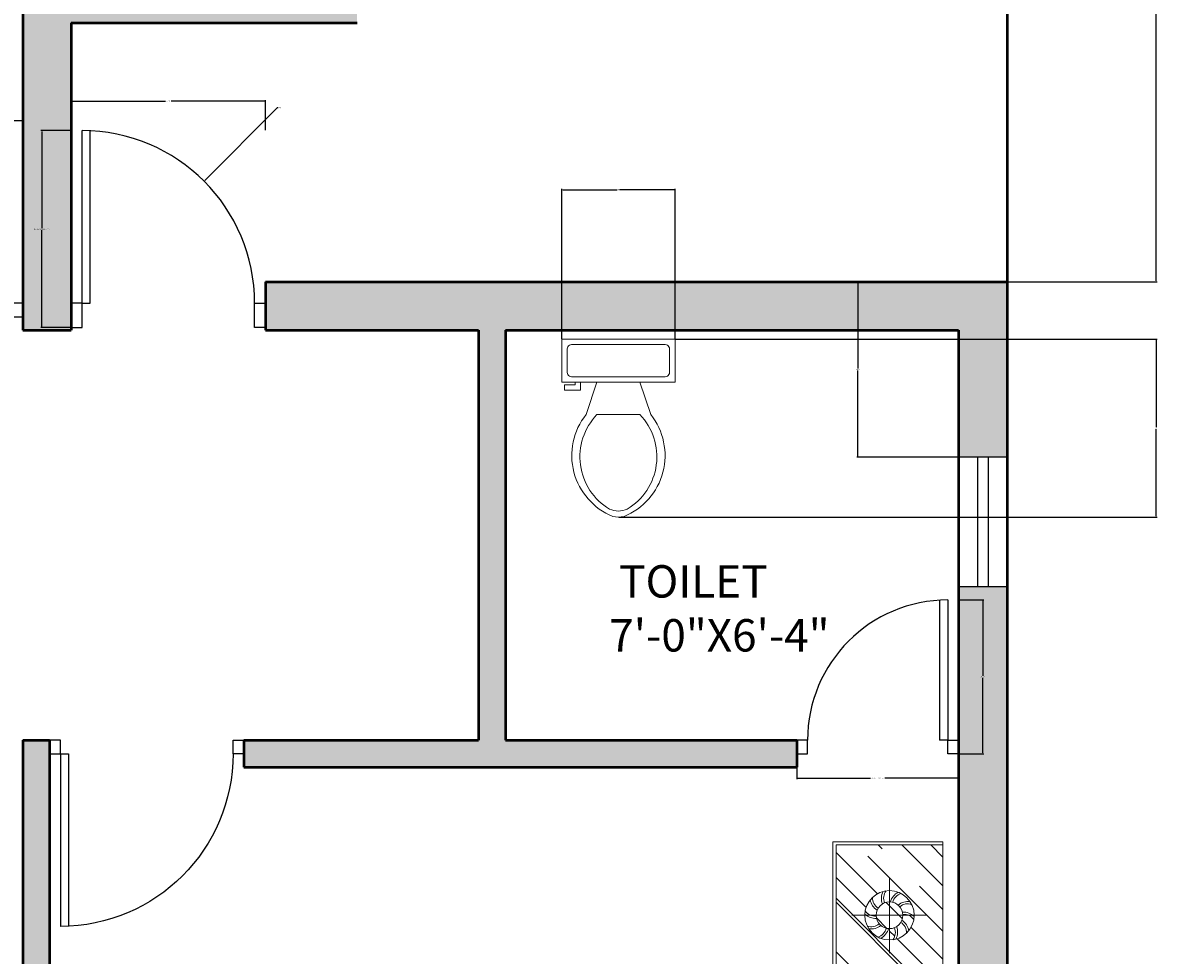
# Model space of a CAD drawing. Units: inches. Extents: x 2831 to 3729, y 3926 to 4974.
# Tile 7 of 8: x 3519 to 3729, y 4672 to 4845. Entities that reach past the tile are written whole.
import ezdxf

# ---------------------------------------------------------------- set-up
doc = ezdxf.new("R2010")
doc.units = ezdxf.units.IN
for name, color, linetype, lineweight in [('A-ANNO-DIMS', 2, 'Continuous', 18), ('A-AREA-IDEN', 7, 'Continuous', 18), ('A-DOOR', 3, 'Continuous', 25), ('A-FLOR-FIXT', 9, 'Continuous', 18), ('A-FURN', 8, 'Continuous', 18), ('A-GLAZ', 4, 'Continuous', 25), ('A-WALL', 7, 'Continuous', 50), ('A-WALL-PATT', 252, 'Continuous', 13)]:
    doc.layers.add(name, color=color, linetype=linetype, lineweight=lineweight)
doc.styles.get("Standard").update_dxf_attribs({"font": 'arial.ttf'})
doc.dimstyles.get("Standard").update_dxf_attribs({"dimtxt": 0.18, "dimasz": 0.18, "dimexe": 0.18, "dimexo": 0.0625, "dimgap": 0.09, "dimtad": 0, "dimtih": 1, "dimtoh": 1, "dimdec": 4, "dimzin": 0, "dimdsep": 46, "dimtxsty": 'Standard', "dimcen": 0.09, "dimadec": 0, "dimazin": 0, "dimtfac": 1, "dimtdec": 4, "dimtofl": 0, "dimtmove": 0, "dimatfit": 3, "dimfxl": 1, "dimtolj": 1, "dimtzin": 0, "dimarcsym": 0})

# ---------------------------------------------------------------- blocks, each defined once
blk = doc.blocks.new('A$C64B41DC1')
for p, q in [((0, 2.5079), (2.9903, 2.5079)), ((0, 2.0879), (0, 2.5079)), ((0.012, 2.4618), (0.0581, 2.5079)), ((0.012, 2.3515), (0.1684, 2.5079)), ((0.012, 2.0999), (0.012, 2.5079)), ((0.0543, 2.2213), (0.3409, 2.5079)), ((0.1689, 2.4179), (0.2589, 2.5079)), ((0.3265, 2.386), (0.4484, 2.5079)), ((0.3699, 2.3332), (0.5445, 2.5079)), ((0.548, 2.5079), (0.548, 2.0999)), ((0.56, 2.5079), (0.56, 2.0879)), ((0.6301, 2.5079), (0.6301, 0.4779)), ((0.6401, 2.461), (0.6401, 2.5079)), ((0.6401, 2.5079), (2.344, 2.5079)), ((2.344, 2.5079), (2.3601, 2.5079)), ((2.344, 2.5079), (2.344, 2.461)), ((2.3601, 2.5079), (2.3601, 2.4761)), ((2.3601, 0.4779), (2.3601, 2.5079)), ((2.4303, 2.5079), (2.4303, 2.0879)), ((2.4423, 2.5079), (2.4423, 2.0999)), ((2.4423, 2.3333), (2.6169, 2.5079)), ((2.4423, 2.2145), (2.7357, 2.5079)), ((2.4423, 2.404), (2.5354, 2.4971)), ((2.705, 2.398), (2.8149, 2.5079)), ((2.7691, 2.3772), (2.8998, 2.5079)), ((2.7819, 2.3646), (2.9252, 2.5079)), ((2.9783, 2.0999), (2.9783, 2.5079)), ((2.9903, 2.0879), (2.9903, 2.5079)), ((0.2157, 2.0999), (0.548, 2.4322)), ((0.2804, 2.1597), (0.2804, 2.4481)), ((2.344, 2.461), (0.6401, 2.461)), ((0.6601, 2.4461), (1.4951, 2.4461)), ((0.6601, 2.4461), (0.6601, 0.5579)), ((1.4951, 2.4461), (0.6697, 2.4461)), ((2.3301, 2.4461), (1.4951, 2.4461)), ((2.3301, 0.5579), (2.3301, 2.4461)), ((2.7099, 2.1597), (2.7099, 2.4481)), ((0.2299, 2.0999), (0.548, 2.418)), ((0.2311, 2.2906), (0.2937, 2.3532)), ((2.6674, 2.2756), (2.7382, 2.3464)), ((2.7914, 2.1846), (2.9783, 2.3715)), ((0.1362, 2.3039), (0.4246, 2.3039)), ((0.3405, 2.3039), (0.3605, 2.3238)), ((2.8541, 2.3039), (2.5657, 2.3039)), ((2.5849, 2.2779), (2.6158, 2.3088)), ((2.6158, 2.3088), (2.6313, 2.3243)), ((2.7249, 2.3076), (2.7512, 2.3339)), ((2.7746, 2.0999), (2.9783, 2.3036)), ((0.012, 2.261), (0.0275, 2.2765)), ((0.0404, 2.0999), (0.1982, 2.2578)), ((0.2905, 2.2539), (0.3304, 2.2938)), ((2.9144, 2.2312), (2.9783, 2.2951)), ((0.1365, 2.0999), (0.251, 2.2144)), ((0.4194, 2.0999), (0.548, 2.2285)), ((2.4423, 2.1353), (2.5382, 2.2312)), ((2.4918, 2.0999), (2.6366, 2.2447)), ((2.7831, 2.0999), (2.8678, 2.1846)), ((2.8962, 2.0999), (2.9783, 2.182)), ((0.4986, 2.0999), (0.548, 2.1493)), ((0.5127, 2.0999), (0.548, 2.1352)), ((0.56, 2.0879), (0, 2.0879)), ((0.548, 2.0999), (0.012, 2.0999)), ((2.4303, 2.0879), (2.9903, 2.0879)), ((2.4423, 2.0999), (2.9783, 2.0999)), ((2.5172, 2.0999), (2.5269, 2.1096)), ((0.9415, 1.9902), (0.9415, 1.3975)), ((0.9715, 1.9906), (0.9715, 1.4076)), ((1.0015, 1.991), (1.0015, 1.4177)), ((1.0315, 1.9916), (1.0315, 1.4279)), ((2.3349, 1.8678), (0.6613, 1.3029)), ((0.8956, 1.1191), (2.3349, 1.8678)), ((1.6636, 1.6412), (0.6601, 1.6412)), ((1.5748, 1.6112), (0.6601, 1.6112)), ((2.377, 1.295), (2.3822, 1.3891)), ((2.4451, 1.295), (2.4503, 1.3891)), ((2.5105, 1.295), (2.5157, 1.3891)), ((2.5471, 1.295), (2.5524, 1.3891)), ((2.7043, 1.295), (2.7095, 1.3891)), ((2.8653, 1.2966), (2.8688, 1.3861)), ((2.3665, 1.295), (2.3665, 1.3839)), ((2.4032, 1.295), (2.4032, 1.3839)), ((2.4346, 1.295), (2.4346, 1.3839)), ((2.4774, 1.2957), (2.4774, 1.3837)), ((2.5, 1.295), (2.5, 1.3839)), ((2.5367, 1.295), (2.5367, 1.3839)), ((2.5681, 1.295), (2.5681, 1.3839)), ((2.5918, 1.295), (2.5918, 1.3839)), ((2.6346, 1.2957), (2.6346, 1.3837)), ((2.6362, 1.2957), (2.6467, 1.3839)), ((2.6729, 1.295), (2.6624, 1.3839)), ((2.6938, 1.295), (2.6938, 1.3839)), ((2.7127, 1.2957), (2.7232, 1.3839)), ((2.7253, 1.295), (2.7253, 1.3839)), ((2.7494, 1.295), (2.7389, 1.3839)), ((2.7718, 1.295), (2.7718, 1.3839)), ((2.7959, 1.295), (2.7854, 1.3839)), ((2.8146, 1.2957), (2.8146, 1.3837)), ((2.8146, 1.2957), (2.8146, 1.3837)), ((2.8282, 1.295), (2.8282, 1.3839)), ((2.8282, 1.295), (2.8282, 1.3839)), ((2.8523, 1.295), (2.8418, 1.3839)), ((2.8523, 1.295), (2.8418, 1.3839)), ((2.8711, 1.2957), (2.8711, 1.3837)), ((2.8711, 1.2957), (2.8875, 1.3822)), ((2.8765, 1.2958), (2.9132, 1.3758)), ((2.8893, 1.3011), (2.9394, 1.3636)), ((2.8713, 1.2927), (2.954, 1.3315)), ((2.8717, 1.2884), (2.9588, 1.3058)), ((2.3601, 1.2873), (2.8639, 1.2873)), ((2.8639, 1.2873), (2.8639, 0.1018)), ((2.8716, 1.2565), (2.9605, 1.2669)), ((2.8744, 1.2817), (2.9603, 1.2869)), ((2.3601, 1.2233), (2.7999, 1.2233)), ((2.7999, 1.2233), (2.7999, 0.1658)), ((2.8716, 1.2212), (2.9605, 1.2212)), ((2.8723, 1.2489), (2.9603, 1.2489)), ((2.3601, 1.1913), (2.7679, 1.1912)), ((2.7679, 1.1912), (2.7679, 0.1978)), ((2.8716, 1.1947), (2.9605, 1.2052)), ((2.8716, 1.181), (2.9605, 1.1705)), ((2.8723, 1.1872), (2.9603, 1.1872)), ((2.8716, 1.1595), (2.9605, 1.1595)), ((2.8716, 1.133), (2.9605, 1.1435)), ((2.8716, 1.1193), (2.9605, 1.1088)), ((2.8716, 1.1035), (2.9605, 1.093)), ((2.8716, 1.0965), (2.9605, 1.0965)), ((2.8716, 1.086), (2.9657, 1.0913)), ((2.8723, 1.1255), (2.9603, 1.1255)), ((2.8723, 1.0858), (2.9605, 1.0753)), ((2.8716, 1.0756), (2.9605, 1.0756)), ((2.8716, 1.0491), (2.9605, 1.0596)), ((2.8723, 1.0416), (2.9603, 1.0416)), ((2.8716, 1.0354), (2.9605, 1.0249)), ((2.8723, 0.9987), (2.9605, 1.0092)), ((2.8723, 0.985), (2.9605, 0.9745)), ((2.8723, 0.9735), (2.9603, 0.9735)), ((2.8716, 0.9346), (2.9605, 0.9241)), ((2.8723, 0.9408), (2.9603, 0.9408)), ((2.8723, 0.8979), (2.9605, 0.9084)), ((2.8723, 0.8726), (2.9603, 0.8726)), ((2.8723, 0.8505), (2.9603, 0.8505)), ((2.8716, 0.7885), (2.9605, 0.799)), ((2.8716, 0.7818), (2.9657, 0.787)), ((2.8716, 0.7503), (2.9657, 0.7556)), ((2.8723, 0.7571), (2.9605, 0.7466)), ((2.8716, 0.7204), (2.9605, 0.7309)), ((2.8716, 0.6995), (2.9605, 0.6995)), ((2.8716, 0.689), (2.9657, 0.6838)), ((2.8716, 0.6576), (2.9657, 0.6523)), ((2.8716, 0.6471), (2.9605, 0.6471)), ((2.8716, 0.5903), (2.9605, 0.6007)), ((2.882, 0.5582), (2.9657, 0.5536)), ((2.8909, 0.5263), (2.9657, 0.5222)), ((0.6301, 0.4779), (2.3601, 0.4779)), ((0.7101, 0.5079), (2.2801, 0.5079)), ((1.2542, 0.1018), (1.2542, 0.4779)), ((1.3182, 0.1658), (1.3182, 0.4779)), ((1.3502, 0.1978), (1.3502, 0.4779)), ((2.8716, 0.4877), (2.9603, 0.4877)), ((2.8928, 0.5169), (2.9605, 0.5169)), ((1.2465, 0.4625), (1.1576, 0.452)), ((1.2465, 0.4365), (1.1577, 0.4365)), ((2.8716, 0.4625), (2.9605, 0.452)), ((2.8716, 0.4365), (2.9603, 0.4365)), ((1.2465, 0.3746), (1.1576, 0.3851)), ((1.2465, 0.3684), (1.1577, 0.3684)), ((2.8716, 0.3746), (2.9605, 0.3851)), ((2.8716, 0.3684), (2.9603, 0.3684)), ((1.2355, 0.3092), (1.1576, 0.3)), ((1.2285, 0.3357), (1.1577, 0.3357)), ((2.8826, 0.3092), (2.9605, 0.3)), ((2.8896, 0.3357), (2.9603, 0.3357)), ((1.2457, 0.2676), (1.1577, 0.2676)), ((2.8723, 0.2676), (2.9603, 0.2676)), ((1.2457, 0.2423), (1.1576, 0.2319)), ((2.8723, 0.2423), (2.9605, 0.2319)), ((1.2465, 0.1742), (1.1524, 0.169)), ((1.2465, 0.2057), (1.1576, 0.2161)), ((1.2465, 0.1847), (1.1576, 0.1847)), ((2.7679, 0.1978), (1.3502, 0.1978)), ((2.8716, 0.2057), (2.9605, 0.2161)), ((2.8716, 0.1847), (2.9605, 0.1847)), ((2.8716, 0.1742), (2.9657, 0.169)), ((1.2465, 0.1428), (1.1524, 0.1376)), ((1.2465, 0.1334), (1.1524, 0.1281)), ((1.2465, 0.1323), (1.1576, 0.1323)), ((1.2465, 0.1323), (1.1576, 0.1323)), ((2.7999, 0.1658), (1.3182, 0.1658)), ((2.8716, 0.1428), (2.9657, 0.1376)), ((2.8716, 0.1334), (2.9657, 0.1281)), ((2.8716, 0.1323), (2.9605, 0.1323)), ((1.2465, 0.1), (1.1576, 0.1105)), ((1.2465, 0.1229), (1.1588, 0.1168)), ((1.2464, 0.1007), (1.1592, 0.0833)), ((1.2468, 0.0964), (1.1641, 0.0576)), ((1.2288, 0.088), (1.1787, 0.0255)), ((1.2415, 0.0933), (1.2049, 0.0133)), ((1.247, 0.0934), (1.2306, 0.0069)), ((1.2527, 0.0925), (1.2493, 0.003)), ((2.8639, 0.1018), (1.2542, 0.1018)), ((1.2658, 0.0941), (1.2762, 0.0052)), ((1.2899, 0.0941), (1.2899, 0.0052)), ((1.2999, 0.0941), (1.3051, 0)), ((1.3313, 0.0941), (1.3365, 0)), ((1.3523, 0.0941), (1.3575, 0)), ((1.3804, 0.0941), (1.3699, 0.0052)), ((1.4119, 0.0934), (1.4223, 0.0052)), ((1.4485, 0.0941), (1.438, 0.0052)), ((1.48, 0.0941), (1.4852, 0)), ((1.5114, 0.0941), (1.5166, 0)), ((1.5323, 0.0941), (1.5376, 0)), ((1.5638, 0.0941), (1.5638, 0.0105)), ((1.6021, 0.0941), (1.6021, 0.0052)), ((1.6336, 0.0941), (1.6336, 0.0052)), ((1.6702, 0.0941), (1.6702, 0.0052)), ((1.7017, 0.0941), (1.7017, 0.0052)), ((1.7122, 0.0941), (1.7174, 0)), ((1.7445, 0.0934), (1.7445, 0.0054)), ((1.7698, 0.0934), (1.7803, 0.0052)), ((1.8065, 0.0941), (1.796, 0.0052)), ((1.8274, 0.0941), (1.8274, 0.0052)), ((1.8379, 0.0941), (1.8431, 0)), ((1.8746, 0.0941), (1.8798, 0)), ((1.8955, 0.0941), (1.8955, 0.0052)), ((1.906, 0.0941), (1.9113, 0)), ((1.9384, 0.0934), (1.9384, 0.0054)), ((1.9609, 0.0941), (1.9609, 0.0052)), ((1.9636, 0.0934), (1.9741, 0.0052)), ((1.9714, 0.0941), (1.9766, 0)), ((1.9976, 0.0941), (1.9976, 0.0052)), ((2.0081, 0.0941), (2.0133, 0)), ((2.029, 0.0941), (2.029, 0.0052)), ((2.0395, 0.0941), (2.0447, 0)), ((2.0797, 0.0941), (2.0797, 0.0052)), ((2.0902, 0.0941), (2.0954, 0)), ((2.1216, 0.0941), (2.1269, 0)), ((2.1412, 0.0941), (2.1412, 0.0052)), ((2.1517, 0.0941), (2.1569, 0)), ((2.1831, 0.0941), (2.1884, 0)), ((2.2093, 0.0941), (2.2093, 0.0052)), ((2.2198, 0.0941), (2.225, 0)), ((2.2512, 0.0941), (2.2565, 0)), ((2.2603, 0.0934), (2.2707, 0.0052)), ((2.2969, 0.0941), (2.2864, 0.0052)), ((2.3089, 0.0934), (2.3193, 0.0052)), ((2.3455, 0.0941), (2.3351, 0.0052)), ((2.3665, 0.0941), (2.3665, 0.0052)), ((2.377, 0.0941), (2.3822, 0)), ((2.4032, 0.0941), (2.4032, 0.0052)), ((2.4346, 0.0941), (2.4346, 0.0052)), ((2.4451, 0.0941), (2.4503, 0)), ((2.4774, 0.0934), (2.4774, 0.0054)), ((2.5, 0.0941), (2.5, 0.0052)), ((2.5105, 0.0941), (2.5157, 0)), ((2.5367, 0.0941), (2.5367, 0.0052)), ((2.5471, 0.0941), (2.5524, 0)), ((2.5681, 0.0941), (2.5681, 0.0052)), ((2.5918, 0.0941), (2.5918, 0.0052)), ((2.6346, 0.0934), (2.6346, 0.0054)), ((2.6362, 0.0934), (2.6467, 0.0052)), ((2.6729, 0.0941), (2.6624, 0.0052)), ((2.6938, 0.0941), (2.6938, 0.0052)), ((2.7043, 0.0941), (2.7095, 0)), ((2.7127, 0.0934), (2.7232, 0.0052)), ((2.7253, 0.0941), (2.7253, 0.0052)), ((2.7494, 0.0941), (2.7389, 0.0052)), ((2.7718, 0.0941), (2.7718, 0.0052)), ((2.7959, 0.0941), (2.7854, 0.0052)), ((2.8146, 0.0934), (2.8146, 0.0054)), ((2.8282, 0.0941), (2.8282, 0.0052)), ((2.8523, 0.0941), (2.8418, 0.0052)), ((2.8653, 0.0925), (2.8688, 0.003)), ((2.8711, 0.0934), (2.8875, 0.0069)), ((2.8713, 0.0964), (2.954, 0.0576)), ((2.8716, 0.1229), (2.9593, 0.1168)), ((2.8717, 0.1007), (2.9588, 0.0833)), ((2.8744, 0.1074), (2.9603, 0.1022)), ((2.8765, 0.0933), (2.9132, 0.0133)), ((2.8893, 0.088), (2.9394, 0.0255))]:
    blk.add_line(p, q)
at = {"ltscale": 10}
for p, q in [((1.4859, 1.5812), (0.6601, 1.5812)), ((1.397, 1.5512), (0.6601, 1.5512))]:
    blk.add_line(p, q, dxfattribs=at)
for centre, radius in [((0.2804, 2.3039), 0.0942), ((2.7099, 2.3039), 0.0942), ((0.2804, 2.3039), 0.051), ((2.7099, 2.3039), 0.051)]:
    blk.add_circle(centre, radius)
for centre, radius, start, end in [((0.6601, 2.4761), 0.03, 180, 270), ((2.3301, 2.4761), 0.03, 270, 0), ((0.2887, 2.3745), 0.0605, 172.17, 218.4897), ((0.2828, 2.3731), 0.0462, 160.3002, 220.538), ((0.3286, 2.3561), 0.0605, 136.17, 182.4897), ((0.3231, 2.3585), 0.0462, 124.3002, 184.538), ((2.6672, 2.3585), 0.0462, 355.462, 55.6998), ((2.6617, 2.3561), 0.0605, 357.5103, 43.83), ((2.7075, 2.3731), 0.0462, 319.462, 19.6998), ((2.7016, 2.3745), 0.0605, 321.5103, 7.83), ((0.2417, 2.3614), 0.0462, 196.3002, 256.538), ((0.3501, 2.3178), 0.0605, 100.17, 146.4897), ((0.347, 2.323), 0.0462, 88.3002, 148.538), ((1.0526, 2.3302), 0.3085, 175.3048, 198.6942), ((-0.8702, 2.0941), 1.6364, 4.8098, 9.1892), ((0.8579, 2.6278), 0.2948, 247.5179, 264.267), ((0.728, 2.111), 0.245, 40.4189, 85.9871), ((1.0164, 5.7096), 3.3803, 266.8134, 276.1602), ((1.3963, 2.1044), 0.245, 94.0129, 139.5811), ((1.1858, 2.3288), 0.1943, 306.5711, 5.89), ((1.5348, 2.2652), 0.1767, 151.7736, 201.6983), ((1.6986, 2.3355), 0.1943, 174.11, 233.4289), ((1.1481, 2.2311), 0.3783, 353.4947, 19.1867), ((1.6871, 3.192), 0.8561, 257.7438, 273.6284), ((1.4882, 2.111), 0.245, 40.4189, 85.9871), ((1.8674, 1.9709), 0.3878, 68.2026, 108.9817), ((2.1269, 2.1044), 0.245, 94.0129, 139.5811), ((2.0342, 2.4856), 0.1563, 261.5958, 298.9092), ((1.9165, 2.3288), 0.1943, 333.7371, 5.89), ((2.6058, 2.2028), 0.517, 163.6046, 172.3273), ((2.6433, 2.323), 0.0462, 31.462, 91.6998), ((2.6402, 2.3178), 0.0605, 33.5103, 79.83), ((2.7486, 2.3614), 0.0462, 283.462, 343.6998), ((0.2457, 2.3659), 0.0605, 208.17, 254.4897), ((0.3449, 2.2742), 0.0605, 64.17, 110.4897), ((0.3455, 2.2802), 0.0462, 52.3002, 112.538), ((0.3151, 2.2419), 0.0605, 28.17, 74.4897), ((2.6448, 2.2802), 0.0462, 67.462, 127.6998), ((2.6454, 2.2742), 0.0605, 69.5103, 115.83), ((2.6752, 2.2419), 0.0605, 105.5103, 151.83), ((2.7446, 2.3659), 0.0605, 285.5103, 331.83), ((0.2153, 2.3276), 0.0462, 232.3002, 292.538), ((0.2158, 2.3336), 0.0605, 244.17, 290.4897), ((0.2138, 2.2848), 0.0462, 268.3002, 328.538), ((0.2107, 2.29), 0.0605, 280.17, 326.4897), ((0.2377, 2.2493), 0.0462, 304.3002, 4.538), ((0.2322, 2.2517), 0.0605, 316.17, 2.4897), ((0.2779, 2.2347), 0.0462, 340.3002, 40.538), ((0.272, 2.2333), 0.0605, 352.17, 38.4897), ((0.3191, 2.2464), 0.0462, 16.3002, 76.538), ((2.6712, 2.2464), 0.0462, 103.462, 163.6998), ((2.7182, 2.2333), 0.0605, 141.5103, 187.83), ((2.7123, 2.2347), 0.0462, 139.462, 199.6998), ((2.7581, 2.2517), 0.0605, 177.5103, 223.83), ((2.7526, 2.2493), 0.0462, 175.462, 235.6998), ((2.7796, 2.29), 0.0605, 213.5103, 259.83), ((2.7765, 2.2848), 0.0462, 211.462, 271.6998), ((2.7744, 2.3336), 0.0605, 249.5103, 295.83), ((2.775, 2.3276), 0.0462, 247.462, 307.6998), ((0.7274, 2.2013), 0.0446, 314.4736, 42.1713), ((-1.6008, 2.277), 2.3618, 357.3905, 358.8876), ((1.9165, 2.3288), 0.1943, 320.9404, 333.7371), ((2.1347, 2.2313), 0.0459, 165.3506, 223.2684), ((0.2688, 2.0945), 0.4956, 344.0243, 8.7071), ((1.204, 2.1778), 0.1681, 337.017, 7.5368), ((1.5671, 2.1546), 0.0547, 142.0833, 220.902), ((1.9346, 2.1778), 0.1681, 337.017, 7.5368), ((0.9385, 1.978), 0.1943, 126.5711, 185.89), ((1.1858, 1.9714), 0.1943, 4.3181, 53.4289), ((1.7059, 1.9714), 0.204, 127.1197, 175.09), ((1.9394, 1.991), 0.1651, 351.2621, 55.7572), ((1.5415, 2.0969), 0.1834, 175.2233, 196.23), ((1.1965, 2.0983), 0.3299, 343.7954, 3.5554), ((2.4617, 2.0719), 0.3745, 173.8296, 196.4356), ((1.2687, 1.9248), 0.1223, 33.628, 86.4744), ((2.2748, 2.5795), 0.6373, 238.3499, 254.3137), ((0.7246, 18.8439), 16.8552, 270.17399, 272.05214), ((1.3401, 1.9404), 0.0603, 49.0991, 101.3702), ((1.7676, 1.0629), 0.9631, 69.6507, 105.9631), ((2.0911, 2.0123), 0.0478, 179.7727, 283.8018), ((0.7417, 2.0149), 0.057, 273.4709, 328.5412), ((0.728, 2.2025), 0.245, 274.0129, 278.3417), ((1.0747, 1.2871), 0.1871, 14.1863, 69.1212), ((1.0274, 1.1334), 0.2527, 40.629, 104.3712), ((0.7347, 1.1553), 0.1649, 347.3109, 116.4454), ((0.7101, 0.5579), 0.05, 180, 270), ((2.2801, 0.5579), 0.05, 270, 0)]:
    blk.add_arc(centre, radius, start, end)
for centre, major_axis, ratio, start_param, end_param in [((1.9938, 1.6262), (0, -0.7531), 0.68, 0.797284, 0.954936), ((2.0643, 1.466), (0, -0.5322), 0.68, 7.239912, 7.311536), ((1.9052, 1.7397), (0, -0.9842), 0.68, 0.74745, 0.979724), ((2.7455, 1.3081), (0, 0.3614), 0.68, 1.900046, 2.742661), ((2.7868, 1.3081), (0, 0.3614), 0.68, 1.900046, 2.614747), ((2.8372, 1.3081), (0, 0.3614), 0.68, 1.900046, 2.479658), ((2.8607, 1.3211), (0, 0.3614), 0.68, 1.938265, 2.479658), ((2.8057, 1.2079), (0, -0.1524), 0.68, 4.821745, 5.895886), ((2.4665, 0.8216), (0, -0.2664), 0.68, 2.006169, 3.565187), ((2.4513, 0.5069), (0, 0.502), 0.68, 5.095327, 6.553458), ((2.7862, 0.8069), (0, -0.2615), 0.68, 3.244645, 4.205018), ((2.7784, 0.8289), (0, -0.1802), 0.68, 3.227058, 4.318474), ((2.396, 0.6032), (0, 0.3641), 0.68, -1.3172, 0.145284), ((2.7821, 0.7971), (0, -0.1589), 0.68, 3.272942, 4.229533), ((2.3507, 0.5642), (0.0073, 0.3819), 0.56205, -1.21172, -0.009991), ((2.2964, 0.5771), (0, -0.3263), 0.68, 1.938944, 2.850232), ((2.0403, 1.6015), (0, -0.8763), 0.68, 6.849801, 6.887077), ((2.4005, 0.7132), (0, -0.1214), 0.68, 2.284368, 3.652258), ((2.3834, 0.7081), (0, 0.1147), 0.68, 4.593909, 6.585576), ((2.3961, 0.7628), (0, -0.0317), 0.68, 1.462497, 5.046281), ((2.3774, 0.7653), (0, -0.0593), 0.68, 5.841311, 7.755362), ((1.9938, 1.1295), (-0.0678, 0.7439), 0.610498, 3.917146, 4.063997), ((2.0643, 0.9693), (0, -0.5322), 0.68, 7.239912, 7.336618), ((1.9052, 1.243), (0, -0.9842), 0.68, 0.74745, 0.979724), ((2.7455, 0.8114), (-0.0599, 0.3735), 0.695517, 1.775813, 2.548612), ((2.7868, 0.8114), (0, 0.3614), 0.68, 1.900046, 2.614747), ((2.8607, 0.8243), (0, 0.3614), 0.68, 1.938265, 2.479658), ((2.4665, 0.3249), (0, -0.2664), 0.68, 2.006169, 3.565187), ((2.7862, 0.3102), (0, -0.2615), 0.68, 3.244645, 4.205018), ((2.4513, 0.0102), (0, 0.502), 0.68, 5.095327, 6.553458), ((1.242, 0.9693), (0, -0.5322), 0.68, 6.586764, 6.677612), ((1.1714, 1.1295), (-0.1157, 0.7241), 0.59432, 3.291697, 3.50733), ((1.0828, 1.243), (0, -0.9842), 0.68, 0.565948, 0.680366), ((1.5283, 0.0674), (0, -0.3703), 0.68, 1.930561, 3.464283), ((1.5736, 0.1065), (0, 0.3641), 0.68, -1.3172, 0.476403), ((1.6289, 0.0102), (0, 0.502), 0.68, 6.655152, 6.661293), ((1.6289, 0.0102), (0, 0.502), 0.68, 5.095327, 5.911219), ((1.6442, 0.3249), (0, -0.2664), 0.68, 2.006169, 2.182797), ((1.9638, 0.3102), (0, -0.2615), 0.68, 4.015924, 4.205018), ((1.956, 0.3322), (0, -0.1802), 0.68, 3.770744, 4.318474), ((2.0606, 0.5616), (0, -0.1803), 0.68, 5.194792, 5.929328), ((2.0606, 0.5616), (0, -0.1803), 0.68, 5.194792, 6.723255), ((2.1315, 0.6603), (0, -0.3155), 0.68, 5.328638, 6.949396), ((2.0549, 0.5656), (0, -0.1303), 0.68, 5.450951, 6.054641), ((2.0643, 0.9693), (0, -0.5322), 0.68, 6.20013, 6.677612), ((1.9938, 1.1295), (-0.0678, 0.7439), 0.610498, 3.199135, 3.592282), ((1.9052, 1.243), (0, -0.9842), 0.68, 0.565948, 0.680366), ((2.3507, 0.0674), (0, -0.3703), 0.68, 1.930561, 3.464283), ((2.396, 0.1065), (0, 0.3641), 0.68, -1.3172, 0.476403), ((2.4513, 0.0102), (0, 0.502), 0.68, 6.655152, 6.661293), ((2.7784, 0.3322), (0, -0.1802), 0.68, 3.227058, 4.318474), ((1.9597, 0.3004), (0, -0.1589), 0.68, 3.14258, 4.229533), ((2.7821, 0.3004), (0, -0.1589), 0.68, 3.272942, 4.229533), ((1.1933, 0.9181), (0, -0.624), 0.68, 0.378672, 0.625379), ((1.3091, 0.6603), (0, -0.3155), 0.68, 6.475719, 6.949396), ((1.1911, 1.1066), (0, 0.8458), 0.68, 3.421828, 3.728616), ((1.474, 0.0804), (0, -0.3263), 0.68, 1.938944, 3.339184), ((2.0157, 0.9181), (0, -0.624), 0.68, -0.280078, 0.625379), ((2.0135, 1.1066), (0, 0.8458), 0.68, 2.978727, 3.728616), ((2.2964, 0.0804), (0, -0.3263), 0.68, 1.938944, 3.339184), ((1.2179, 1.1047), (0, -0.8763), 0.68, 6.507006, 6.887077), ((1.5781, 0.2165), (0, -0.1214), 0.68, 2.284368, 3.726131), ((2.0403, 1.1047), (0, -0.8763), 0.68, 6.099302, 6.887077), ((2.4005, 0.2165), (0, -0.1214), 0.68, 2.284368, 3.726131), ((1.555, 0.2685), (0, -0.0593), 0.68, 3.732151, 7.755362), ((1.561, 0.2114), (0, 0.1147), 0.68, 4.593909, 6.647252), ((2.3774, 0.2685), (0, -0.0593), 0.68, 3.732151, 7.755362), ((2.3834, 0.2114), (0, 0.1147), 0.68, 4.593909, 6.647252), ((1.5737, 0.2661), (0, -0.0317), 0.68, 1.462497, 5.046281), ((2.3961, 0.2661), (0, -0.0317), 0.68, 1.462497, 5.046281)]:
    blk.add_ellipse(centre, major_axis=major_axis, ratio=ratio, start_param=start_param, end_param=end_param)
blk = doc.blocks.new('*U8')
for p, q in [((9.5, -6), (9.5, -2)), ((-8, -8.5), (-8, -8)), ((-7, -8), (-7, -9.5)), ((-4, -8), (-6, -14)), ((4, -8), (6, -14)), ((-10, -8.5), (-8, -8.5)), ((-10, -9.5), (-10, -8.5)), ((-7, -9.5), (-10, -9.5)), ((4, -14), (-4, -14))]:
    blk.add_line(p, q)
blk.add_lwpolyline([(10.5, -8), (10.5, 0), (-10.5, 0), (-10.5, -8)], close=True)
for points in [[(-9.5, -2), (-9.5, -6)], [(8.5, -1), (-8.5, -1)], [(-8.5, -7), (8.5, -7)]]:
    blk.add_lwpolyline(points)
for centre, radius, start, end in [((-8.62, -1.88), 0.884, 81.8699, 188.1301), ((8.62, -1.88), 0.884, 351.8699, 98.1301), ((-8.62, -6.12), 0.884, 171.8699, 278.1301), ((8.62, -6.12), 0.884, 261.8699, 8.1301), ((3.52, -21.58), 12.17, 141.4691, 247.9714), ((4.2, -21.82), 11.33, 136.3677, 238.9468), ((-3.52, -21.58), 12.17, 292.0284, 38.5307), ((-4.2, -21.82), 11.33, 301.053, 43.6321), ((0, -27.88), 4, 245.7318, 294.2682), ((0, -29), 4, 254.8605, 285.1395)]:
    blk.add_arc(centre, radius, start, end)
blk = doc.blocks.new('DOOR-SWING-32IN')
for p, q in [((-32, 2.5), (-34, 2.5)), ((-32, 0), (-32, 2.5)), ((0, 0), (0, 2.5)), ((0, 2.5), (2, 2.5)), ((-34, 0), (-32, 0)), ((2, 0), (0, 0)), ((-1.5, 0), (-1.5, -31.96)), ((0, 0), (-1.5, 0)), ((0, 0), (0, -32))]:
    blk.add_line(p, q)
blk.add_arc((0, 0), 32, 180, 270)
blk = doc.blocks.new('DOOR-SWING-26IN')
for p, q in [((-1.5, 25.96), (-1.5, 0)), ((0, 26), (0, 0)), ((-26, 0), (-28, 0)), ((-26, -2.5), (-26, 0)), ((0, 0), (-1.5, 0)), ((0, -2.5), (0, 0)), ((0, 0), (2, 0)), ((-28, -2.5), (-26, -2.5)), ((2, -2.5), (0, -2.5))]:
    blk.add_line(p, q)
blk.add_arc((0, 0), 26, 90, 180)
blk = doc.blocks.new('DOOR-SWING-32IN-DEEP-JAMB')
for p, q in [((0, 0), (0, 32)), ((1.5, 0), (1.5, 31.96)), ((0, 0), (-2, 0)), ((0, -4.5), (0, 0)), ((0, 0), (1.5, 0)), ((32, -4.5), (32, 0)), ((32, 0), (34, 0)), ((-2, -4.5), (0, -4.5)), ((34, -4.5), (32, -4.5))]:
    blk.add_line(p, q)
blk.add_arc((0, 0), 32, 0, 90)
blk = doc.blocks.new('WINDOW-24IN-PLAN')
for p, q in [((0, 24), (9, 24)), ((3.5, 0), (3.5, 24)), ((5.5, 0), (5.5, 24)), ((0, 0), (9, 0))]:
    blk.add_line(p, q)
blk = doc.blocks.new('*D19')
at = {"layer": 'A-ANNO-DIMS', "color": 0, "lineweight": -2, "transparency": 16777216}
for p, q in [((3662.31, 4709.58), (3662.31, 4704.96)), ((3692.31, 4709.58), (3692.31, 4704.96)), ((3662.49, 4705.14), (3676, 4705.14)), ((3692.13, 4705.14), (3678.62, 4705.14))]:
    blk.add_line(p, q, dxfattribs=at)
at = {"layer": 'A-ANNO-DIMS', "color": 0, "transparency": 16777216}
for points in [[(3662.49, 4705.17), (3662.49, 4705.11), (3662.31, 4705.14)], [(3692.13, 4705.17), (3692.13, 4705.11), (3692.31, 4705.14)]]:
    blk.add_solid(points, dxfattribs=at)
at = {"layer": 'Defpoints', "color": 0, "transparency": 16777216}
for p in [(3662.31, 4709.64), (3692.31, 4709.64), (3692.31, 4705.14)]:
    blk.add_point(p, dxfattribs=at)
at = {"layer": 'A-ANNO-DIMS', "color": 0, "transparency": 16777216, "insert": (3677.31, 4705.14), "char_height": 0.18, "attachment_point": 5}
blk.add_mtext('\\A1;BATH DOOR 30 TYP.', dxfattribs=at)
blk = doc.blocks.new('*D20')
at = {"layer": 'A-ANNO-DIMS', "color": 0, "lineweight": -2, "transparency": 16777216}
for p, q in [((3692.37, 4738.14), (3696.99, 4738.14)), ((3696.81, 4737.96), (3696.81, 4724.07)), ((3696.81, 4709.82), (3696.81, 4723.71)), ((3692.37, 4709.64), (3696.99, 4709.64))]:
    blk.add_line(p, q, dxfattribs=at)
at = {"layer": 'A-ANNO-DIMS', "color": 0, "transparency": 16777216}
for points in [[(3696.78, 4737.96), (3696.84, 4737.96), (3696.81, 4738.14)], [(3696.78, 4709.82), (3696.84, 4709.82), (3696.81, 4709.64)]]:
    blk.add_solid(points, dxfattribs=at)
at = {"layer": 'Defpoints', "color": 0, "transparency": 16777216}
for p in [(3692.31, 4738.14), (3696.81, 4738.14), (3692.31, 4709.64)]:
    blk.add_point(p, dxfattribs=at)
at = {"layer": 'A-ANNO-DIMS', "color": 0, "transparency": 16777216, "insert": (3696.81, 4723.89), "char_height": 0.18, "attachment_point": 5}
blk.add_mtext('\\A1;29 TYP.', dxfattribs=at)
blk = doc.blocks.new('*D21')
at = {"layer": 'A-ANNO-DIMS', "color": 0, "lineweight": -2, "transparency": 16777216}
for p, q in [((3527.75, 4825.14), (3522.15, 4825.14)), ((3522.33, 4824.96), (3522.33, 4807.07)), ((3522.33, 4788.82), (3522.33, 4806.71)), ((3527.75, 4788.64), (3522.15, 4788.64))]:
    blk.add_line(p, q, dxfattribs=at)
at = {"layer": 'A-ANNO-DIMS', "color": 0, "transparency": 16777216}
for points in [[(3522.3, 4824.96), (3522.36, 4824.96), (3522.33, 4825.14)], [(3522.3, 4788.82), (3522.36, 4788.82), (3522.33, 4788.64)]]:
    blk.add_solid(points, dxfattribs=at)
at = {"layer": 'Defpoints', "color": 0, "transparency": 16777216}
for p in [(3522.33, 4825.14), (3527.81, 4825.14), (3527.81, 4788.64)]:
    blk.add_point(p, dxfattribs=at)
at = {"layer": 'A-ANNO-DIMS', "color": 0, "transparency": 16777216, "insert": (3522.33, 4806.89), "char_height": 0.18, "attachment_point": 5}
blk.add_mtext('\\A1;DEEP JAMB DOOR 37 TYP.', dxfattribs=at)
blk = doc.blocks.new('*D22')
at = {"layer": 'A-ANNO-DIMS', "color": 0, "lineweight": -2, "transparency": 16777216}
for p, q in [((3527.81, 4825.2), (3527.81, 4830.8)), ((3527.99, 4830.62), (3545.28, 4830.62)), ((3563.63, 4830.62), (3546.34, 4830.62)), ((3563.81, 4825.2), (3563.81, 4830.8))]:
    blk.add_line(p, q, dxfattribs=at)
at = {"layer": 'A-ANNO-DIMS', "color": 0, "transparency": 16777216}
for points in [[(3527.99, 4830.65), (3527.99, 4830.59), (3527.81, 4830.62)], [(3563.63, 4830.65), (3563.63, 4830.59), (3563.81, 4830.62)]]:
    blk.add_solid(points, dxfattribs=at)
at = {"layer": 'Defpoints', "color": 0, "transparency": 16777216}
for p in [(3563.81, 4830.62), (3527.81, 4825.14), (3563.81, 4825.14)]:
    blk.add_point(p, dxfattribs=at)
at = {"layer": 'A-ANNO-DIMS', "color": 0, "transparency": 16777216, "insert": (3545.81, 4830.62), "char_height": 0.18, "attachment_point": 5}
blk.add_mtext('\\A1;36 TYP.', dxfattribs=at)
blk = doc.blocks.new('*D32')
at = {"layer": 'A-ANNO-DIMS', "color": 0, "lineweight": -2, "transparency": 16777216}
for p, q in [((3499.8, 4934.24), (3519.1, 4934.24)), ((3518.92, 4934.06), (3518.92, 4880.81)), ((3518.92, 4827.2), (3518.92, 4880.45)), ((3499.8, 4827.02), (3519.1, 4827.02))]:
    blk.add_line(p, q, dxfattribs=at)
at = {"layer": 'A-ANNO-DIMS', "color": 0, "transparency": 16777216}
for points in [[(3518.89, 4934.06), (3518.95, 4934.06), (3518.92, 4934.24)], [(3518.89, 4827.2), (3518.95, 4827.2), (3518.92, 4827.02)]]:
    blk.add_solid(points, dxfattribs=at)
at = {"layer": 'Defpoints', "color": 0, "transparency": 16777216}
for p in [(3499.74, 4934.24), (3518.92, 4934.24), (3499.74, 4827.02)]:
    blk.add_point(p, dxfattribs=at)
at = {"layer": 'A-ANNO-DIMS', "color": 0, "transparency": 16777216, "insert": (3518.92, 4880.63), "char_height": 0.18, "attachment_point": 5}
blk.add_mtext('\\A1;107', dxfattribs=at)
blk = doc.blocks.new('*D57')
at = {"layer": 'A-ANNO-DIMS', "color": 0, "lineweight": -2, "transparency": 16777216}
for p, q in [((3701.37, 4946.14), (3729.14, 4946.14)), ((3728.96, 4945.96), (3728.96, 4871.82)), ((3728.96, 4797.32), (3728.96, 4871.46)), ((3701.37, 4797.14), (3729.14, 4797.14))]:
    blk.add_line(p, q, dxfattribs=at)
at = {"layer": 'A-ANNO-DIMS', "color": 0, "transparency": 16777216}
for points in [[(3728.93, 4945.96), (3728.99, 4945.96), (3728.96, 4946.14)], [(3728.93, 4797.32), (3728.99, 4797.32), (3728.96, 4797.14)]]:
    blk.add_solid(points, dxfattribs=at)
at = {"layer": 'Defpoints', "color": 0, "transparency": 16777216}
for p in [(3701.31, 4946.14), (3728.96, 4946.14), (3701.31, 4797.14)]:
    blk.add_point(p, dxfattribs=at)
at = {"layer": 'A-ANNO-DIMS', "color": 0, "transparency": 16777216, "insert": (3728.96, 4871.64), "char_height": 0.18, "attachment_point": 5}
blk.add_mtext('\\A1;149', dxfattribs=at)
blk = doc.blocks.new('*D59')
at = {"layer": 'A-ANNO-DIMS', "color": 0, "lineweight": -2, "transparency": 16777216}
for p, q in [((3701.25, 4797.14), (3673.48, 4797.14)), ((3673.66, 4796.96), (3673.66, 4781.05)), ((3673.66, 4764.77), (3673.66, 4780.69)), ((3701.25, 4764.59), (3673.48, 4764.59))]:
    blk.add_line(p, q, dxfattribs=at)
at = {"layer": 'A-ANNO-DIMS', "color": 0, "transparency": 16777216}
for points in [[(3673.63, 4796.96), (3673.69, 4796.96), (3673.66, 4797.14)], [(3673.63, 4764.77), (3673.69, 4764.77), (3673.66, 4764.59)]]:
    blk.add_solid(points, dxfattribs=at)
at = {"layer": 'Defpoints', "color": 0, "transparency": 16777216}
for p in [(3673.66, 4797.14), (3701.31, 4797.14), (3701.31, 4764.59)]:
    blk.add_point(p, dxfattribs=at)
at = {"layer": 'A-ANNO-DIMS', "color": 0, "transparency": 16777216, "insert": (3673.66, 4780.87), "char_height": 0.18, "attachment_point": 5}
blk.add_mtext('\\A1;32.546', dxfattribs=at)
blk = doc.blocks.new('*D60')
at = {"layer": 'A-ANNO-DIMS', "color": 0, "lineweight": -2, "transparency": 16777216}
for p, q in [((3618.75, 4786.56), (3618.75, 4814.33)), ((3618.93, 4814.15), (3629.05, 4814.15)), ((3639.57, 4814.15), (3629.45, 4814.15)), ((3639.75, 4786.56), (3639.75, 4814.33))]:
    blk.add_line(p, q, dxfattribs=at)
at = {"layer": 'A-ANNO-DIMS', "color": 0, "transparency": 16777216}
for points in [[(3618.93, 4814.18), (3618.93, 4814.12), (3618.75, 4814.15)], [(3639.57, 4814.18), (3639.57, 4814.12), (3639.75, 4814.15)]]:
    blk.add_solid(points, dxfattribs=at)
at = {"layer": 'Defpoints', "color": 0, "transparency": 16777216}
for p in [(3639.75, 4814.15), (3618.75, 4786.5), (3639.75, 4786.5)]:
    blk.add_point(p, dxfattribs=at)
at = {"layer": 'A-ANNO-DIMS', "color": 0, "transparency": 16777216, "insert": (3629.25, 4814.15), "char_height": 0.18, "attachment_point": 5}
blk.add_mtext('\\A1;21', dxfattribs=at)
blk = doc.blocks.new('*D61')
at = {"layer": 'A-ANNO-DIMS', "color": 0, "lineweight": -2, "transparency": 16777216}
for p, q in [((3639.81, 4786.5), (3729.14, 4786.5)), ((3728.96, 4786.32), (3728.96, 4770.18)), ((3728.96, 4753.68), (3728.96, 4769.82)), ((3629.31, 4753.5), (3729.14, 4753.5))]:
    blk.add_line(p, q, dxfattribs=at)
at = {"layer": 'A-ANNO-DIMS', "color": 0, "transparency": 16777216}
for points in [[(3728.93, 4786.32), (3728.99, 4786.32), (3728.96, 4786.5)], [(3728.93, 4753.68), (3728.99, 4753.68), (3728.96, 4753.5)]]:
    blk.add_solid(points, dxfattribs=at)
at = {"layer": 'Defpoints', "color": 0, "transparency": 16777216}
for p in [(3639.75, 4786.5), (3629.25, 4753.5), (3728.96, 4753.5)]:
    blk.add_point(p, dxfattribs=at)
at = {"layer": 'A-ANNO-DIMS', "color": 0, "transparency": 16777216, "insert": (3728.96, 4770), "char_height": 0.18, "attachment_point": 5}
blk.add_mtext('\\A1;33', dxfattribs=at)
blk = doc.blocks.new('*D80')
at = {"layer": 'A-ANNO-DIMS', "color": 0, "lineweight": -2, "transparency": 16777216}
for p, q in [((3566.01, 4829.34), (3552.56, 4815.9)), ((3566.19, 4829.34), (3566.01, 4829.34)), ((3529.72, 4793.14), (3529.9, 4793.14)), ((3529.81, 4793.05), (3529.81, 4793.23))]:
    blk.add_line(p, q, dxfattribs=at)
at = {"layer": 'A-ANNO-DIMS', "color": 0, "transparency": 16777216}
blk.add_solid([(3552.54, 4815.92), (3552.58, 4815.87), (3552.44, 4815.77)], dxfattribs=at)
at = {"layer": 'Defpoints', "color": 0, "transparency": 16777216}
for p in [(3552.44, 4815.77), (3529.81, 4793.14)]:
    blk.add_point(p, dxfattribs=at)
at = {"layer": 'A-ANNO-DIMS', "color": 0, "transparency": 16777216, "insert": (3566.5, 4829.34), "char_height": 0.18, "attachment_point": 5}
blk.add_mtext('\\A1;R32', dxfattribs=at)

msp = doc.modelspace()

# ---------------------------------------------------------------- hatches: boundary and pattern name
at = {"layer": 'A-WALL-PATT'}
h = msp.add_hatch(color=256, dxfattribs=at)
h.dxf.hatch_style = 1
h.paths.add_polyline_path([(3580.8091, 4946.1405), (3557.3091, 4946.1405), (3557.3091, 4937.1405), (3571.8091, 4937.1405), (3571.8091, 4854.1405), (3523.8091, 4854.1405), (3523.8091, 4907.1405), (3518.8091, 4907.1405), (3518.8091, 4788.1405), (3527.8091, 4788.1405), (3527.8091, 4845.1405), (3580.8091, 4845.1405)])
h = msp.add_hatch(color=256, dxfattribs=at)
h.dxf.hatch_style = 1
h.paths.add_polyline_path([(3662.3091, 4712.1405), (3608.3091, 4712.1405), (3608.3091, 4788.1405), (3692.3091, 4788.1405), (3692.3091, 4764.594), (3701.3091, 4764.594), (3701.3091, 4797.1405), (3563.8091, 4797.1405), (3563.8091, 4788.1405), (3603.3091, 4788.1405), (3603.3091, 4712.1405), (3559.8091, 4712.1405), (3559.8091, 4707.1405), (3662.3091, 4707.1405)])
h = msp.add_hatch(color=256, dxfattribs=at)
h.dxf.hatch_style = 1
h.paths.add_polyline_path([(3701.3091, 4740.594), (3692.3091, 4740.594), (3692.3091, 4707.1405), (3692.3091, 4535.1405), (3656.0591, 4535.1405), (3656.0591, 4526.1405), (3701.3091, 4526.1405)])
h = msp.add_hatch(color=256, dxfattribs=at)
h.dxf.hatch_style = 1
h.paths.add_polyline_path([(3523.8091, 4712.1405), (3518.8091, 4712.1405), (3518.8091, 4535.1405), (3514.8091, 4535.1405), (3470.5591, 4535.1405), (3470.5591, 4526.1405), (3560.0591, 4526.1405), (3560.0591, 4535.1405), (3523.8091, 4535.1405)])

# ---------------------------------------------------------------- linework, layer by layer
at = {"layer": 'A-WALL'}
for p, q in [((3701.3091, 4946.1405), (3701.3091, 4466.1405)), ((3518.8091, 4907.1405), (3518.8091, 4788.1405)), ((3527.8091, 4845.1405), (3580.8091, 4845.1405)), ((3527.8091, 4845.1405), (3527.8091, 4788.1405)), ((3563.8091, 4797.1405), (3701.3091, 4797.1405)), ((3563.8091, 4797.1405), (3563.8091, 4788.1405)), ((3518.8091, 4788.1405), (3527.8091, 4788.1405)), ((3563.8091, 4788.1405), (3603.3091, 4788.1405)), ((3603.3091, 4788.1405), (3603.3091, 4712.1405)), ((3608.3091, 4788.1405), (3692.3091, 4788.1405)), ((3608.3091, 4788.1405), (3608.3091, 4712.1405)), ((3692.3091, 4788.1405), (3692.3091, 4707.1405)), ((3518.8091, 4712.1405), (3518.8091, 4535.1405)), ((3518.8091, 4712.1405), (3523.8091, 4712.1405)), ((3523.8091, 4712.1405), (3523.8091, 4535.1405)), ((3559.8091, 4712.1405), (3559.8091, 4707.1405)), ((3559.8091, 4712.1405), (3603.3091, 4712.1405)), ((3608.3091, 4712.1405), (3662.3091, 4712.1405)), ((3662.3091, 4712.1405), (3662.3091, 4707.1405)), ((3559.8091, 4707.1405), (3662.3091, 4707.1405)), ((3692.3091, 4707.1405), (3692.3091, 4535.1405))]:
    msp.add_line(p, q, dxfattribs=at)

# ---------------------------------------------------------------- block references
at = {"layer": 'A-DOOR', "extrusion": (0, 0, -1), "zscale": -1, "rotation": 180}
msp.add_blockref('DOOR-SWING-32IN', (-3516.8091, 4793.1405), dxfattribs=at)
at = {"layer": 'A-DOOR'}
for name, p in [('DOOR-SWING-32IN-DEEP-JAMB', (3529.8091, 4793.1405)), ('DOOR-SWING-26IN', (3690.3091, 4712.1405))]:
    msp.add_blockref(name, p, dxfattribs=at)
at = {"layer": 'A-DOOR', "extrusion": (0, 0, -1), "zscale": -1}
msp.add_blockref('DOOR-SWING-32IN', (-3525.8091, 4709.6405), dxfattribs=at)
at = {"layer": 'A-FLOR-FIXT'}
msp.add_blockref('*U8', (3629.2512, 4786.5016), dxfattribs=at)
at = {"layer": 'A-FURN', "xscale": 48.57198025145115, "yscale": 48.57198025145115, "zscale": 48.57198025145115, "rotation": 270}
msp.add_blockref('A$C64B41DC1', (3567.6073, 4693.324), dxfattribs=at)
at = {"layer": 'A-GLAZ', "rotation": 180}
msp.add_blockref('WINDOW-24IN-PLAN', (3701.3091, 4764.594), dxfattribs=at)

# ---------------------------------------------------------------- texts
at = {"layer": 'A-AREA-IDEN', "insert": (3627.5508, 4744.5932), "char_height": 6, "attachment_point": 1}
msp.add_mtext_dynamic_manual_height_columns(' TOILET\\P7\'-0"X6\'-4"', width=76.299971, gutter_width=12.5, heights=[0], dxfattribs=at)

# ---------------------------------------------------------------- dimensions: what is measured, and where the dimension line sits
at = {"layer": 'A-ANNO-DIMS'}
for base, p1, p2, override, picture, middle in [((3728.9591, 4946.1405), (3701.3091, 4797.1405), (3701.3091, 4946.1405), {"dimdec": 0, "dimlfac": 1, "dimrnd": 0, "dimzin": 0, "dimdsep": 46, "dimlunit": 2}, '*D57', (3728.9591, 4871.6405)), ((3518.9199, 4934.242), (3499.7423, 4827.0157), (3499.7423, 4934.242), {"dimdec": 0, "dimlfac": 1, "dimrnd": 0, "dimzin": 0, "dimdsep": 46, "dimlunit": 2}, '*D32', (3518.9199, 4880.6288)), ((3673.65907, 4797.1405), (3701.30907, 4764.59401), (3701.30907, 4797.14049), {"dimdec": 3, "dimlfac": 1, "dimrnd": 0, "dimzin": 0, "dimdsep": 46, "dimlunit": 2}, '*D59', (3673.65907, 4780.86725)), ((3728.9591, 4753.5016), (3639.7512, 4786.5016), (3629.2512, 4753.5016), {"dimdec": 0, "dimlfac": 1, "dimrnd": 0, "dimzin": 0, "dimdsep": 46, "dimlunit": 2}, '*D61', (3728.9591, 4770.0016))]:
    dim = msp.add_linear_dim(base=base, p1=p1, p2=p2, angle=90, dimstyle='Standard', override=override, dxfattribs=at)
    dim.commit()
    dim.dimension.update_dxf_attribs({"geometry": picture, "text_midpoint": middle})
for base, p1, p2, text, picture, middle in [((3563.8091, 4830.6155), (3527.8091, 4825.1405), (3563.8091, 4825.1405), '<> TYP.', '*D22', (3545.8091, 4830.6155)), ((3692.3091, 4705.1405), (3662.3091, 4709.6405), (3692.3091, 4709.6405), 'BATH DOOR <> TYP.', '*D19', (3677.3091, 4705.1405))]:
    dim = msp.add_linear_dim(base=base, p1=p1, p2=p2, text=text, dimstyle='Standard', override={"dimdec": 0, "dimlfac": 1, "dimrnd": 0, "dimzin": 0, "dimdsep": 46, "dimlunit": 2}, dxfattribs=at)
    dim.commit()
    dim.dimension.update_dxf_attribs({"geometry": picture, "text_midpoint": middle})
dim = msp.add_radius_dim(center=(3529.8091, 4793.1405), mpoint=(3552.4362, 4815.7682), dimstyle='Standard', override={"dimdec": 0, "dimlfac": 1, "dimrnd": 0, "dimzin": 0, "dimdsep": 46, "dimlunit": 2}, dxfattribs=at)
dim.commit()
dim.dimension.update_dxf_attribs({"geometry": '*D80', "text_midpoint": (3566.4966, 4829.3448), "dimtype": 164})
for base, p1, p2, text, picture, middle in [((3522.3340712546, 4825.14049496), (3527.8090712546, 4788.64049496), (3527.8090712546, 4825.14049496), 'DEEP JAMB DOOR <> TYP.', '*D21', (3522.3340712546, 4806.89049496)), ((3696.8090712546, 4738.14049496), (3692.3090712546, 4709.64049496), (3692.3090712546, 4738.14049496), '<> TYP.', '*D20', (3696.8090712546, 4723.89049496))]:
    dim = msp.add_linear_dim(base=base, p1=p1, p2=p2, angle=90, text=text, dimstyle='Standard', override={"dimdec": 0, "dimlfac": 1, "dimrnd": 0, "dimzin": 0, "dimdsep": 46, "dimlunit": 2}, dxfattribs=at)
    dim.commit()
    dim.dimension.update_dxf_attribs({"geometry": picture, "text_midpoint": middle})
dim = msp.add_linear_dim(base=(3639.7512, 4814.1516), p1=(3618.7512, 4786.5016), p2=(3639.7512, 4786.5016), dimstyle='Standard', override={"dimdec": 0, "dimlfac": 1, "dimrnd": 0, "dimzin": 0, "dimdsep": 46, "dimlunit": 2}, dxfattribs=at)
dim.commit()
dim.dimension.update_dxf_attribs({"geometry": '*D60', "text_midpoint": (3629.2512, 4814.1516)})

doc.saveas('drawing.dxf')
